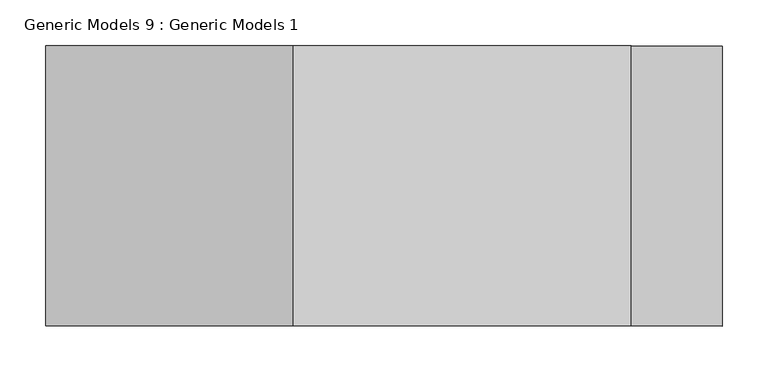
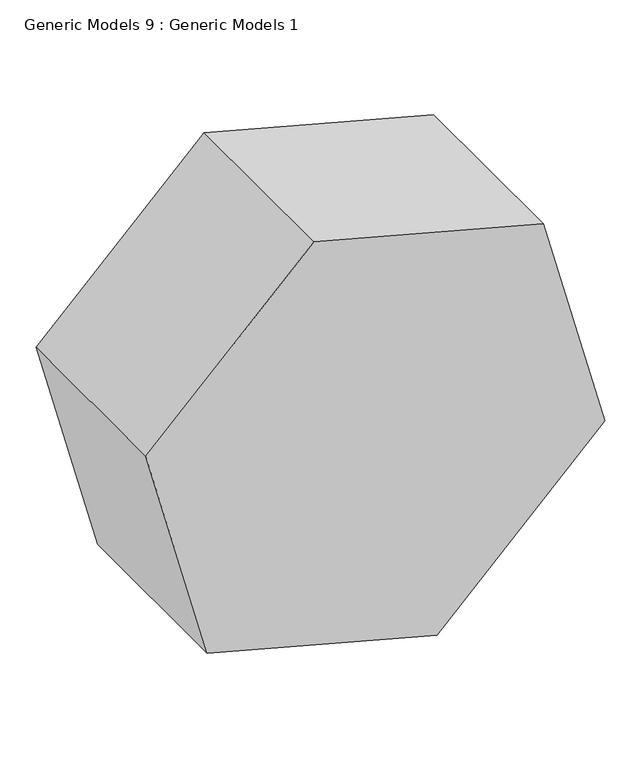
"""IFC4 building model written with IfcOpenShell, lengths in millimetres: proxy geometry, Generic Models 9 : Generic Models 1."""

from ifc_helpers import new_model, si_unit, frame, origin, place, context, project, spatial, polyline, outline, extrude, source, transform, mapped, element, save


def generic_models_9_generic_models_1_cc0d601c(model_context):
    return source(origin(), model_context, "Body", "SweptSolid", [
        extrude(outline(polyline([(904.7566299, 592.2198357), (1003.366686, 224.2020959), (733.9590024, -45.2055877), (365.9412626, 53.4044685), (267.3312064, 421.4222083), (536.73889, 690.8298919), (904.7566299, 592.2198357)])), frame((0.0, -9086.6225464, 0.0), z_axis=(0.0, 1.0, 0.0), x_axis=(0.0, 0.0, 1.0)), (0.0, 0.0, 1.0), 304.8),
    ])


if __name__ == "__main__":
    model = new_model("IFC4")
    model_context = context("Model", 3, world=origin())
    ifc_project = project(units=[si_unit("LENGTHUNIT", "METRE", prefix="MILLI")], contexts=[model_context])
    site = spatial("IfcSite", under=ifc_project)
    building = spatial("IfcBuilding", under=site)
    placement = place(None, origin())
    generic_models_9_generic_models_1_shape = generic_models_9_generic_models_1_cc0d601c(model_context)
    element("IfcBuildingElementProxy", 1, Name="Generic Models 9 : Generic Models 1", ObjectType="Generic Models 9 : Generic Models 1", at=placement, inside=building, context=model_context, shape_type="MappedRepresentation", body=[
        mapped(generic_models_9_generic_models_1_shape, transform((0.0, 0.0, 0.0), x_axis=(1.0, 0.0, 0.0), y_axis=(0.0, 1.0, 0.0), z_axis=(0.0, 0.0, 1.0))),
    ])
    save(model, "model.ifc")

# Revit data of these elements
# Element 1 (IfcBuildingElementProxy, "Generic Models 9 : Generic Models 1")
#   Materials on its faces: "Carpet (1)"
# Materials
#   "Carpet (1)": class "Carpet", colour RGB 124 80 67, transparency 0, Description = "Interior finish", Cost = 0
